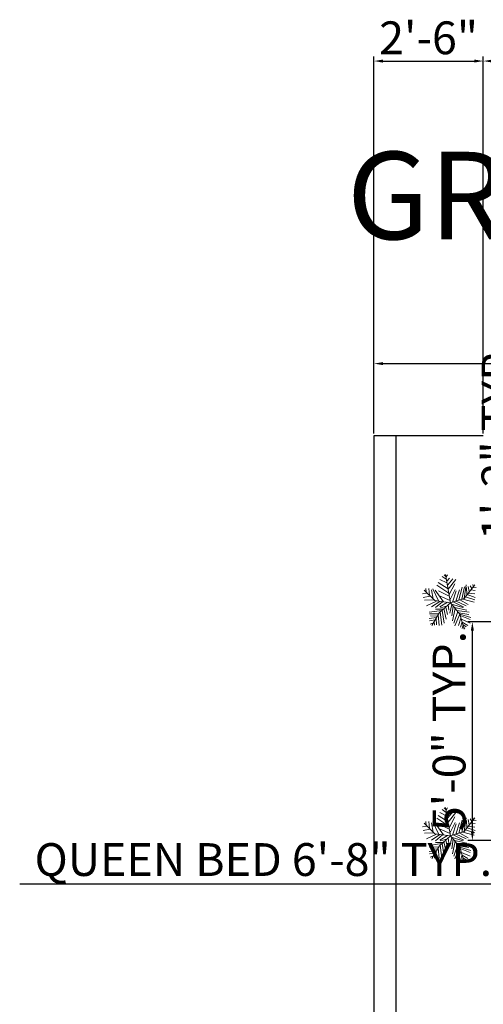
# Model space of a CAD drawing. Units: inches. Extents: x 889 to 1572, y 7262 to 8387.
# Tile 5 of 8: x 889 to 1016, y 8117 to 8387. Entities that reach past the tile are written whole.
import ezdxf

# ---------------------------------------------------------------- set-up
doc = ezdxf.new("R2010")
doc.units = ezdxf.units.IN
for name, color, linetype, lineweight in [('A-ANNO-DIMS', 2, 'Continuous', 18), ('A-ANNO-TITL', 7, 'Continuous', 35), ('C-SITE', 7, 'Continuous', 30), ('L-PLNT', 94, 'Continuous', 13)]:
    doc.layers.add(name, color=color, linetype=linetype, lineweight=lineweight)
doc.styles.get("Standard").update_dxf_attribs({"font": 'arial.ttf'})
doc.dimstyles.new('ISO-25', dxfattribs={"dimtxt": 9, "dimasz": 2.5, "dimexe": 1.25, "dimexo": 0.625, "dimtad": 1, "dimlunit": 3, "dimtxsty": 'Standard', "dimcen": 2.5, "dimadec": 0, "dimazin": 0, "dimtfac": 1, "dimtmove": 0, "dimatfit": 3, "dimfxl": 1, "dimarcsym": 0})

# ---------------------------------------------------------------- blocks, each defined once
blk = doc.blocks.new('*U15')
for p, q in [((-5.114, 28.097), (-24.676, 40.636)), ((-7.288, 39.707), (-21.778, 46.673)), ((-8.737, 47.138), (-17.069, 52.711)), ((-10.186, 53.64), (-13.084, 55.962)), ((0, 0), (-10.5, 57)), ((-9.099, 51.782), (-6.563, 55.962)), ((-7.65, 43.423), (-2.578, 49.46)), ((-5.839, 35.992), (4.667, 48.067)), ((-5.114, 27.632), (10.463, 46.673)), ((-47.498, 19.737), (-55.83, 18.344)), ((-31.5, 4.5), (-52.5, 25.5)), ((-48.585, 21.131), (-49.309, 29.026)), ((-43.513, 28.561), (-42.427, 15.558)), ((-38.442, 26.239), (-34.819, 7.663)), ((-35.544, 28.097), (-24.314, 3.947)), ((-14.533, 2.09), (-30.834, 25.31)), ((-3.665, 19.273), (-27.574, 35.527)), ((-24.314, 23.917), (-2.941, 13.7)), ((-2.941, 16.486), (8.652, 37.85)), ((-1.129, 6.734), (9.014, 26.704)), ((3.942, 1.625), (11.187, 24.381)), ((10.101, 3.483), (17.708, 26.239)), ((16.259, 5.805), (23.142, 31.348)), ((22.055, 7.198), (27.489, 32.277)), ((27, 9), (48, 36)), ((27.127, 9.056), (31.112, 35.992)), ((31.836, 30.883), (32.561, 16.486)), ((35.096, 32.741), (37.27, 22.524)), ((36.183, 19.737), (48.137, 17.88)), ((38.719, 34.134), (41.979, 28.561)), ((40.53, 25.775), (48.862, 24.846)), ((43.791, 29.954), (51.036, 30.883)), ((44.153, 36.456), (45.239, 32.741)), ((-40.615, 13.7), (-55.105, 10.913)), ((-33.37, 6.269), (-52.207, 5.34)), ((-28.299, 3.483), (-47.86, -5.805)), ((-21.416, 3.018), (-38.079, -8.128)), ((0, 0), (-31.5, 4.5)), ((-15.982, 2.09), (-30.11, -9.521)), ((0, 0), (-22.5, -19.5)), ((-6.563, 1.161), (-21.416, -8.128)), ((-20.691, 13.7), (-1.129, 4.876)), ((0, 0), (27, 9)), ((0, 0), (18, -22.5)), ((6.478, 1.625), (26.04, -8.592)), ((11.187, 3.483), (30.749, -5.805)), ((18.07, 5.805), (35.096, -3.483)), ((24.229, 7.663), (46.688, 1.625)), ((29.662, 12.307), (48.137, 6.269)), ((33.285, 16.486), (48.862, 10.913)), ((-17.431, -15.094), (-42.789, -18.809)), ((-22.5, -19.5), (-37.5, -45)), ((-15.257, -12.772), (-30.11, -12.772)), ((-20.691, -18.345), (-17.793, -44.352)), ((-6.563, -5.805), (-19.967, -9.985)), ((-17.069, -15.094), (-12.721, -40.172)), ((-13.446, -11.378), (-8.737, -32.741)), ((-9.461, -8.592), (-6.201, -23.453)), ((-4.752, -3.483), (-3.665, -14.629)), ((2.493, -3.019), (-1.491, -20.202)), ((1.769, -2.555), (24.229, -9.521)), ((5.029, -6.27), (2.131, -25.775)), ((9.014, -11.378), (3.58, -35.992)), ((14.085, -16.951), (6.478, -40.172)), ((7.565, -9.056), (32.198, -14.629)), ((12.274, -15.094), (36.907, -18.809)), ((-28.299, -29.026), (-42.789, -31.348)), ((-24.314, -21.596), (-42.427, -22.06)), ((-30.834, -34.135), (-42.427, -35.528)), ((-26.849, -26.24), (-40.253, -25.775)), ((-32.646, -36.921), (-31.921, -44.352)), ((-29.023, -30.884), (-27.936, -43.887)), ((-25.038, -23.918), (-22.865, -45.281)), ((18.07, -22.524), (8.289, -45.745)), ((20.244, -30.419), (15.897, -44.816)), ((16.259, -19.738), (36.183, -22.989)), ((18, -22.5), (27, -52.5)), ((18.433, -22.524), (40.53, -29.026)), ((19.157, -25.311), (38.719, -33.206)), ((22.78, -37.85), (19.519, -48.532)), ((21.331, -32.741), (39.081, -40.636)), ((22.78, -38.314), (34.372, -44.816)), ((-34.457, -39.708), (-40.978, -42.494)), ((24.591, -45.745), (23.142, -50.854)), ((24.591, -43.423), (30.749, -47.603)), ((26.764, -49.925), (28.213, -50.854))]:
    blk.add_line(p, q)
blk = doc.blocks.new('*D28')
at = {"layer": 'A-ANNO-DIMS', "color": 0, "lineweight": -2, "transparency": 16777216}
for p, q in [((986.05, 8273.36), (986.05, 8293.82)), ((1466.05, 8273.36), (1466.05, 8293.82)), ((988.55, 8292.57), (1463.55, 8292.57))]:
    blk.add_line(p, q, dxfattribs=at)
at = {"layer": 'A-ANNO-DIMS', "color": 0, "transparency": 16777216}
for points in [[(988.55, 8292.98), (988.55, 8292.15), (986.05, 8292.57)], [(1463.55, 8292.98), (1463.55, 8292.15), (1466.05, 8292.57)]]:
    blk.add_solid(points, dxfattribs=at)
at = {"layer": 'Defpoints', "color": 0, "transparency": 16777216}
for p in [(1466.05, 8292.57), (986.05, 8272.73), (1466.05, 8272.73)]:
    blk.add_point(p, dxfattribs=at)
at = {"layer": 'A-ANNO-DIMS', "color": 0, "transparency": 16777216, "insert": (1226.05, 8297.79), "char_height": 9, "attachment_point": 5}
blk.add_mtext("40'", dxfattribs=at)
blk = doc.blocks.new('*D43')
at = {"layer": 'A-ANNO-DIMS', "color": 0, "lineweight": -2, "transparency": 16777216}
for p, q in [((1025.05, 8161.11), (1025.05, 8148.48)), ((1105.05, 8161.11), (1105.05, 8148.48)), ((1025.05, 8149.73), (888.91, 8149.73)), ((1102.55, 8149.73), (1027.55, 8149.73))]:
    blk.add_line(p, q, dxfattribs=at)
at = {"layer": 'A-ANNO-DIMS', "color": 0, "transparency": 16777216}
for points in [[(1027.55, 8150.15), (1027.55, 8149.31), (1025.05, 8149.73)], [(1102.55, 8150.15), (1102.55, 8149.31), (1105.05, 8149.73)]]:
    blk.add_solid(points, dxfattribs=at)
at = {"layer": 'Defpoints', "color": 0, "transparency": 16777216}
for p in [(1025.05, 8161.73), (1105.05, 8161.73), (1025.05, 8149.73)]:
    blk.add_point(p, dxfattribs=at)
at = {"layer": 'A-ANNO-DIMS', "color": 0, "transparency": 16777216, "insert": (955.73, 8155.29), "char_height": 9, "attachment_point": 5}
blk.add_mtext('QUEEN BED 6\'-8" TYP.', dxfattribs=at)
blk = doc.blocks.new('*D44')
at = {"layer": 'A-ANNO-DIMS', "color": 0, "lineweight": -2, "transparency": 16777216}
for p, q in [((1024.42, 8221.73), (1011.8, 8221.73)), ((1013.05, 8164.23), (1013.05, 8219.23)), ((1024.42, 8161.73), (1011.8, 8161.73))]:
    blk.add_line(p, q, dxfattribs=at)
at = {"layer": 'A-ANNO-DIMS', "color": 0, "transparency": 16777216}
for points in [[(1012.63, 8219.23), (1013.47, 8219.23), (1013.05, 8221.73)], [(1012.63, 8164.23), (1013.47, 8164.23), (1013.05, 8161.73)]]:
    blk.add_solid(points, dxfattribs=at)
at = {"layer": 'Defpoints', "color": 0, "transparency": 16777216}
for p in [(1013.05, 8221.73), (1025.05, 8221.73), (1025.05, 8161.73)]:
    blk.add_point(p, dxfattribs=at)
at = {"layer": 'A-ANNO-DIMS', "color": 0, "transparency": 16777216, "insert": (1007.83, 8191.73), "char_height": 9, "attachment_point": 5, "rotation": 90}
blk.add_mtext('5\'-0" TYP.', dxfattribs=at)
blk = doc.blocks.new('*D54')
at = {"layer": 'A-ANNO-DIMS', "color": 0, "lineweight": -2, "transparency": 16777216}
for p, q in [((1026.37, 8241.45), (1026.37, 8299.22)), ((1027.85, 8241.45), (1025.12, 8241.45)), ((1026.37, 8229.95), (1026.37, 8238.95)), ((1027.85, 8227.45), (1025.12, 8227.45))]:
    blk.add_line(p, q, dxfattribs=at)
at = {"layer": 'A-ANNO-DIMS', "color": 0, "transparency": 16777216}
for points in [[(1025.96, 8238.95), (1026.79, 8238.95), (1026.37, 8241.45)], [(1025.96, 8229.95), (1026.79, 8229.95), (1026.37, 8227.45)]]:
    blk.add_solid(points, dxfattribs=at)
at = {"layer": 'Defpoints', "color": 0, "transparency": 16777216}
for p in [(1026.37, 8241.45), (1028.47, 8241.45), (1028.47, 8227.45)]:
    blk.add_point(p, dxfattribs=at)
at = {"layer": 'A-ANNO-DIMS', "color": 0, "transparency": 16777216, "insert": (1021.23, 8271.58), "char_height": 9, "attachment_point": 5, "rotation": 90}
blk.add_mtext('1\'-2" TYP.', dxfattribs=at)
blk = doc.blocks.new('*D71')
at = {"layer": 'A-ANNO-DIMS', "color": 0, "lineweight": -2, "transparency": 16777216}
for p, q in [((986.05, 8273.36), (986.05, 8376.85)), ((988.55, 8375.6), (1013.55, 8375.6)), ((1016.05, 8273.36), (1016.05, 8376.85))]:
    blk.add_line(p, q, dxfattribs=at)
at = {"layer": 'A-ANNO-DIMS', "color": 0, "transparency": 16777216}
for points in [[(988.55, 8376.02), (988.55, 8375.18), (986.05, 8375.6)], [(1013.55, 8376.02), (1013.55, 8375.18), (1016.05, 8375.6)]]:
    blk.add_solid(points, dxfattribs=at)
at = {"layer": 'Defpoints', "color": 0, "transparency": 16777216}
for p in [(1016.05, 8375.6), (986.05, 8272.73), (1016.05, 8272.73)]:
    blk.add_point(p, dxfattribs=at)
at = {"layer": 'A-ANNO-DIMS', "color": 0, "transparency": 16777216, "insert": (1001.05, 8380.82), "char_height": 9, "attachment_point": 5}
blk.add_mtext('2\'-6"', dxfattribs=at)
blk = doc.blocks.new('*D73')
at = {"layer": 'A-ANNO-DIMS', "color": 0, "lineweight": -2, "transparency": 16777216}
for p, q in [((1016.05, 8273.36), (1016.05, 8376.85)), ((1018.55, 8375.6), (1022.55, 8375.6)), ((1025.05, 8264.36), (1025.05, 8376.85)), ((1025.05, 8375.6), (1052.72, 8375.6))]:
    blk.add_line(p, q, dxfattribs=at)
at = {"layer": 'A-ANNO-DIMS', "color": 0, "transparency": 16777216}
for points in [[(1018.55, 8376.02), (1018.55, 8375.18), (1016.05, 8375.6)], [(1022.55, 8376.02), (1022.55, 8375.18), (1025.05, 8375.6)]]:
    blk.add_solid(points, dxfattribs=at)
at = {"layer": 'Defpoints', "color": 0, "transparency": 16777216}
for p in [(1025.05, 8375.6), (1016.05, 8272.73), (1025.05, 8263.73)]:
    blk.add_point(p, dxfattribs=at)
at = {"layer": 'A-ANNO-DIMS', "color": 0, "transparency": 16777216, "insert": (1040.14, 8380.82), "char_height": 9, "attachment_point": 5}
blk.add_mtext('0\'-9"', dxfattribs=at)

msp = doc.modelspace()

# ---------------------------------------------------------------- linework, layer by layer
at = {"layer": 'C-SITE'}
for p, q in [((986.049, 8272.731), (986.049, 7393.731)), ((1016.049, 8272.731), (986.049, 8272.731)), ((992.049, 8272.731), (992.049, 7405.731))]:
    msp.add_line(p, q, dxfattribs=at)

# ---------------------------------------------------------------- block references
at = {"layer": 'L-PLNT', "xscale": 0.137481440781912, "yscale": 0.137481440781912, "zscale": 0.137481440781912}
for p in [(1007.095, 8226.898), (1007.095, 8162.934)]:
    msp.add_blockref('*U15', p, dxfattribs=at)

# ---------------------------------------------------------------- texts
at = {"layer": 'A-ANNO-TITL', "insert": (978.629, 8350.694), "char_height": 24, "attachment_point": 1}
msp.add_mtext_dynamic_manual_height_columns('GROUND FLOOR HOUSE PLAN', width=625.16453, gutter_width=0, heights=[25.177], dxfattribs=at)

# ---------------------------------------------------------------- dimensions: what is measured, and where the dimension line sits
at = {"layer": 'A-ANNO-DIMS'}
for base, p1, p2, override, picture, middle in [((1016.049, 8375.6), (986.049, 8272.731), (1016.049, 8272.731), {"dimdec": 1, "dimlfac": 1, "dimrnd": 0, "dimzin": 1, "dimdsep": 46, "dimlunit": 4, "dimfrac": 2}, '*D71', (1001.049, 8380.82)), ((1025.049, 8375.6), (1016.049, 8272.731), (1025.049, 8263.731), {"dimdec": 1, "dimlfac": 1, "dimrnd": 0, "dimzin": 1, "dimdsep": 46, "dimlunit": 4, "dimfrac": 2}, '*D73', (1040.136, 8380.82)), ((1466.049, 8292.566), (986.049, 8272.731), (1466.049, 8272.731), {"dimclrd": 0, "dimclre": 0, "dimclrt": 0}, '*D28', (1226.049, 8297.786))]:
    dim = msp.add_linear_dim(base=base, p1=p1, p2=p2, dimstyle='ISO-25', override=override, dxfattribs=at)
    dim.commit()
    dim.dimension.update_dxf_attribs({"geometry": picture, "text_midpoint": middle})
for base, p1, p2, angle, text, picture, middle in [((1026.373, 8241.453), (1028.473, 8227.453), (1028.473, 8241.453), 90, '<> TYP.', '*D54', (1021.227, 8271.585)), ((1013.049, 8221.731), (1025.049, 8161.731), (1025.049, 8221.731), 90, '<> TYP.', '*D44', (1007.828, 8191.731)), ((1025.049, 8149.731), (1105.049, 8161.731), (1025.049, 8161.731), 180, 'QUEEN BED <> TYP.', '*D43', (955.728, 8155.286))]:
    dim = msp.add_linear_dim(base=base, p1=p1, p2=p2, angle=angle, text=text, dimstyle='ISO-25', override={"dimdec": 1, "dimlfac": 1, "dimrnd": 0, "dimzin": 1, "dimdsep": 46, "dimlunit": 4, "dimfrac": 2}, dxfattribs=at)
    dim.commit()
    dim.dimension.update_dxf_attribs({"geometry": picture, "text_midpoint": middle})

doc.saveas('drawing.dxf')
